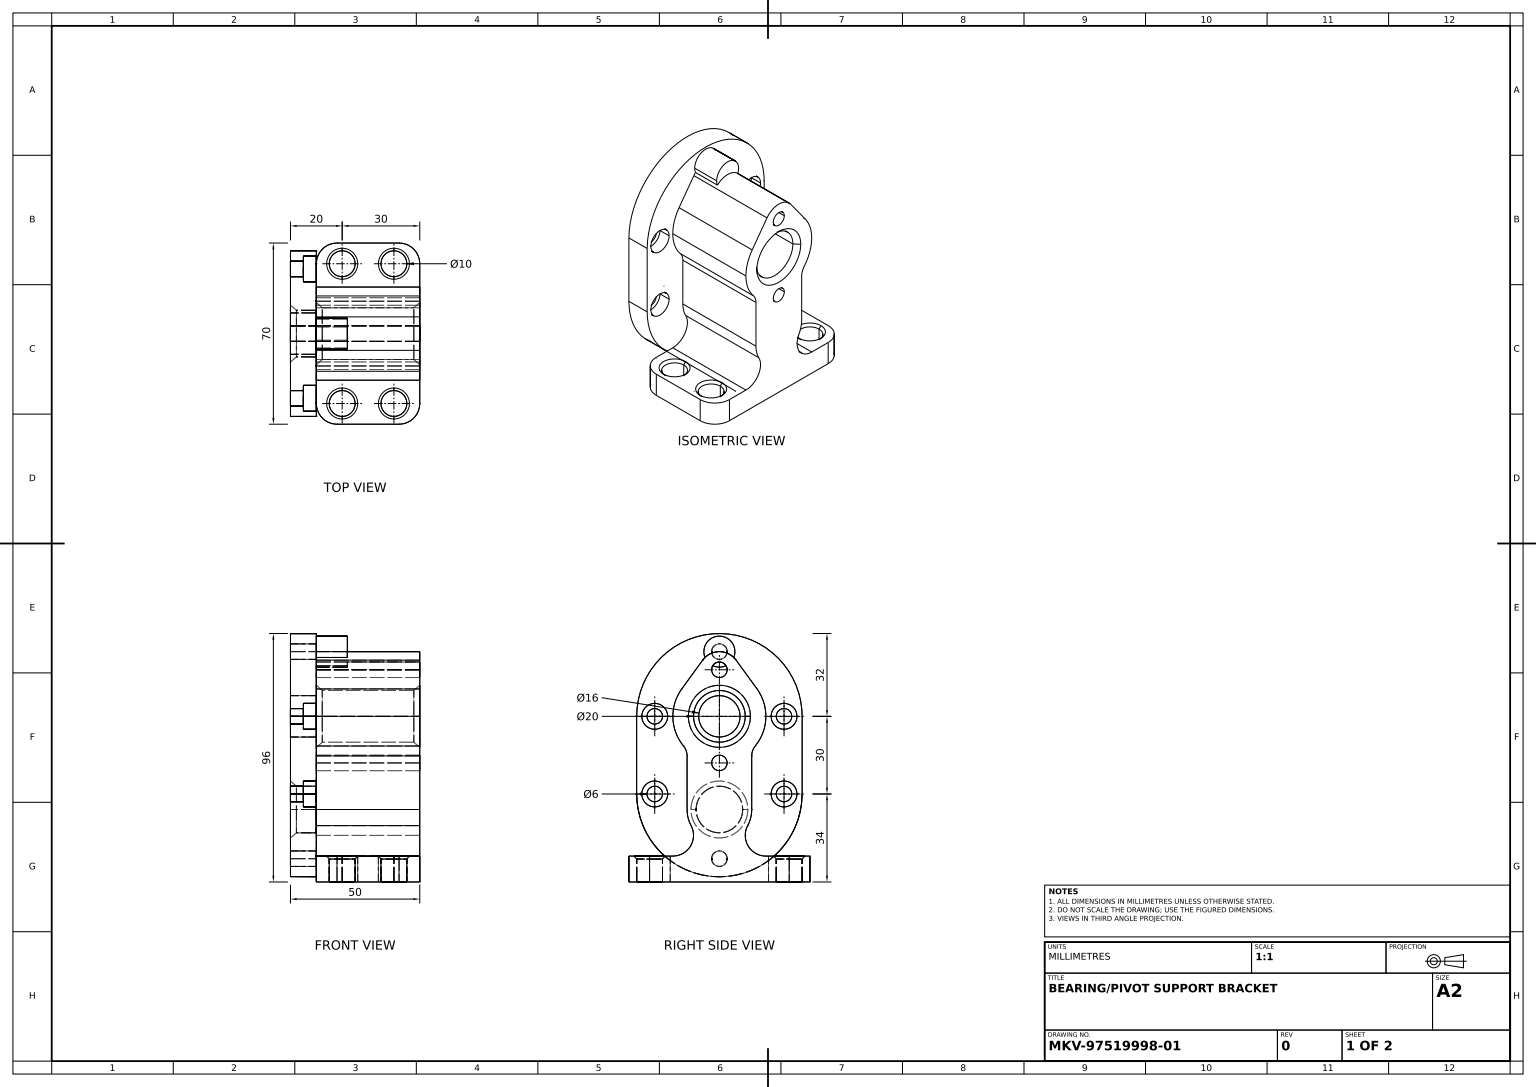
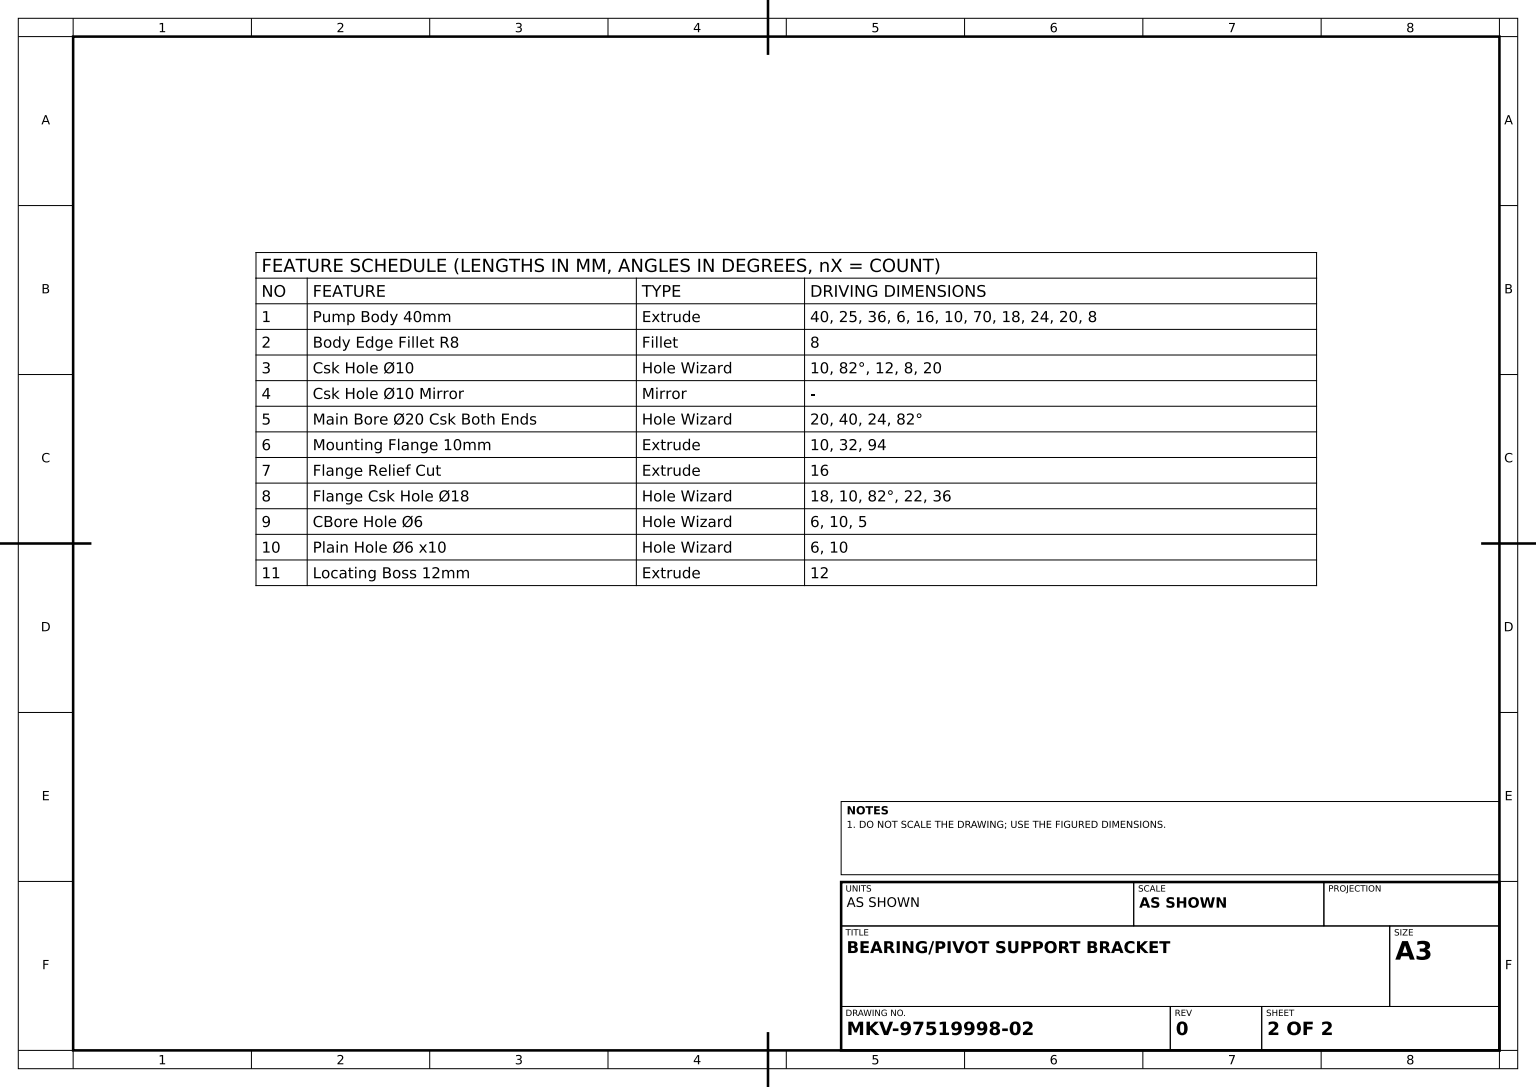
SolidWorks part; units mm, degrees
material "Plain Carbon Steel"
ref_plane "Front Plane" through (0, 0, 0) normal (0, 0, 1) x (1, 0, 0)
ref_plane "Top Plane" through (0, 0, 0) normal (0, 1, 0) x (1, 0, 0)
ref_plane "Right Plane" through (0, 0, 0) normal (1, 0, 0) x (0, 0, -1)
sketch "Body Profile Sketch" plane through (0, 0, 0) normal (1, 0, 0) x (0, 0, -1)
  line L0 (-12.5, -15.2889) -> (-12.5, -36)
  line L1 (12.5, -15.2889) -> (12.5, -36)
  line L2 (0, 0) -> (0, -6.2857) construction
  line L3 (-18, -54) -> (-35, -54)
  line L4 (-35, -54) -> (-35, -64)
  line L5 (-35, -64) -> (35, -64)
  line L6 (35, -64) -> (35, -54)
  line L7 (35, -54) -> (18, -54)
  line L8 (-14.5564, 10.5882) -> (-6.4695, 21.7059)
  line L9 (14.5564, 10.5882) -> (6.4695, 21.7059)
  arc A0 (13.875, -11.4667) -> (14.5564, 10.5882) centre (0, 0) ccw
  arc A1 (-12.5, -15.2889) -> (-13.875, -11.4667) centre (-18.5, -15.2889) ccw
  arc A2 (12.5, -15.2889) -> (13.875, -11.4667) centre (18.5, -15.2889) cw
  arc A3 (6.4695, 21.7059) -> (-6.4695, 21.7059) centre (0, 17) ccw
  arc A8 (-14.5564, 10.5882) -> (-13.875, -11.4667) centre (0, 0) ccw
  circle A10 centre (0, -36) radius 10 construction
  arc A11 (-12.5, -36) -> (-10.9412, -42.2353) centre (0.75, -36) ccw
  circle A12 centre (0, -36) radius 12 construction
  arc A13 (-18, -54) -> (-10.9412, -42.2353) centre (-18, -46) ccw
  arc A14 (12.5, -36) -> (10.9412, -42.2353) centre (-0.75, -36) cw
  arc A15 (18, -54) -> (10.9412, -42.2353) centre (18, -46) cw
  circle A16 centre (0, -18) radius 3
  circle A17 centre (0, 18) radius 3
  point P14 (0, 25)
  point P15 (0, -64)
  dimension "D1" = 18
  dimension "D4" = 6
  dimension "D5" = 16
  dimension "D8" = 24
  dimension "D9" = 25
  dimension "D11" = 20
  dimension "D12" = 8
  dimension "D13" = 6
  dimension "D15" = 6
  dimension "D2" = 25
  dimension "D3" = 36
  dimension "D6" = 10
  dimension "D7" = 70
  dimension "D10" = 18
  dimension "D14" = 18
  dimension "D16" = 18
  dimension "D17" = 36
extrude "Pump Body 40mm" add sketch "Body Profile Sketch" along normal blind 40
fillet "Body Edge Fillet R8" radius 8 4 edges at (0, -59, 35) (40, -59, 35) (0, -59, -35) (40, -59, -35)
hole_wizard "Csk Hole Ø10" positions "3DSketch2" profile "Sketch3" legacy end condition up to next
sketch3d "3DSketch2"
  line L1 (10, -54, 27) -> (52.0975, -54, 27) construction
  line L3 (32, -54, 35) -> (8, -54, 35) construction
  line L4 (40, -54, 18) -> (40, -54, 27) construction
  point P0 (10, -54, 27)
  point P2 (30, -54, 27)
  dimension "D1" = 8
  dimension "D2" = 20
  dimension "D3" = 10
sketch "Sketch3" plane through (10, -54, 27) normal (1, 0, 0) x (0, 0, 1)
  line L0 (0, 0) -> (0, 10)
  line L1 (0, 10) -> (5, 10)
  line L2 (5, 10) -> (5, 1.1504)
  line L3 (5, 1.1504) -> (6, 0)
  line L4 (6, 0) -> (0, 0)
  line L5 (0, -6.4453) -> (0, 115.525) construction
  line L6 (-5, 1.1504) -> (-6, 0) construction
  dimension "Diameter" = 10
  dimension "Depth" = 10
  dimension "C-Sink Angle" = 82
  dimension "C-Sink Diameter" = 12
mirror "Csk Hole Ø10 Mirror" about plane through (0, 0, 0) normal (0, 0, 1) of "Csk Hole Ø10"
hole_wizard "Main Bore Ø20 Csk Both Ends" positions "3DSketch3" profile "Sketch7" hole size "Ø20.0" standard "ISO" end condition up to next
sketch3d "3DSketch3"
  arc A3 (40, -11.4667, -13.875) -> (40, 10.5882, -14.5564) centre (40, 0, 0) ccw construction
  point P0 (0, 0, 0)
  point P3 (40, 0, 0)
  point P21 (58, 0, 0)
sketch "Sketch7" plane through (40, 0, 0) normal (0, 1, 0) x (0, 0, -1)
  line L0 (0, 0) -> (0, 40)
  line L1 (0, 40) -> (12, 40)
  line L2 (10, 37.6993) -> (10, 2.3007)
  line L3 (10, 2.3007) -> (12, 0)
  line L5 (12, 0) -> (0, 0)
  line L6 (-10, 2.3007) -> (-12, 0) construction
  line L7 (12, 40) -> (10, 37.6993)
  line L8 (-12, 40) -> (-10, 37.6993) construction
  line L11 (0, -6.35) -> (0, 107.95) construction
  dimension "Thru Hole Dia." = 20
  dimension "Thru Hole Depth" = 40
  dimension "Near C'Sink Dia." = 24
  dimension "Near C'Sink Angle" = 82
  dimension "Far C'Sink Dia." = 24
  dimension "Far C'Sink Angle" = 82
sketch "Mounting Flange Sketch" plane through (0, 0, 0) normal (-1, 0, 0) x (0, 0, 1)
  line L0 (0, 0) -> (0, -30) construction
  line L1 (32, 0) -> (32, -30)
  line L2 (-32, 0) -> (-32, -30)
  arc A0 (32, 0) -> (-32, 0) centre (0, 0) ccw
  arc A1 (-32, -30) -> (32, -30) centre (0, -30) ccw
  point P4 (0, -15)
  point P9 (0, 32)
  point P10 (0, -62)
  dimension "D2" = 32
  dimension "D1" = 94
extrude "Mounting Flange 10mm" add sketch "Mounting Flange Sketch" along normal blind 10
sketch "Flange Relief Cut Sketch" plane through (-10, 0, 0) normal (-1, 0, 0) x (0, 0, 1)
  circle A0 centre (0, 0) radius 8
  dimension "D1" = 16
extrude "Flange Relief Cut" cut sketch "Flange Relief Cut Sketch" against normal up to next
hole_wizard "Flange Csk Hole Ø18" positions "3DSketch4" profile "Sketch9" legacy
sketch3d "3DSketch4"
  line L1 (-10, -62, 0) -> (-10, 32, 0) construction
  line L2 (-10, 0, -32) -> (-10, 0, 32) construction
  arc A1 (-10, -30, -32) -> (-10, -30, 32) centre (-10, -30, 0) ccw construction
  arc A2 (-10, 0, 32) -> (-10, 0, -32) centre (-10, 0, 0) ccw construction
  point P0 (-10, -36, 0)
  point P17 (-42, -30, 0)
  point P21 (-42, 0, 0)
  dimension "D1" = 36
sketch "Sketch9" plane through (-10, -36, 0) normal (0, 1, 0) x (0, 0, 1)
  line L0 (0, 0) -> (0, 9.798)
  line L1 (0, 9.798) -> (9, 9.798)
  line L2 (9, 9.798) -> (9, 2.3007)
  line L3 (9, 2.3007) -> (11, 0)
  line L4 (11, 0) -> (0, 0)
  line L5 (0, -6.4453) -> (0, 115.525) construction
  line L6 (-9, 2.3007) -> (-11, 0) construction
  dimension "Diameter" = 18
  dimension "Depth" = 10
  dimension "C-Sink Angle" = 82
  dimension "C-Sink Diameter" = 22
sketch "Small Hole Layout Sketch" plane through (0, 0, 0) normal (-1, 0, 0) x (0, 0, 1)
  line L0 (0, 0) -> (0, -30) construction
  line L1 (25, 0) -> (25, -30)
  line L2 (-25, 0) -> (-25, -30)
  line L3 (32, 0) -> (32, -30) construction
  line L4 (11, -36) -> (0, -36) construction
  arc A0 (25, 0) -> (-25, 0) centre (0, 0) ccw
  arc A1 (-25, -30) -> (25, -30) centre (0, -30) ccw
  point P3 (0, -15)
  point P10 (32, -15)
  point P11 (0, 25)
  point P13 (0, -55)
  dimension "D1" = 19
hole_wizard "CBore Hole Ø6" positions "3DSketch6" profile "Sketch15" legacy end condition through all
sketch3d "3DSketch6"
  point P0 (0, -30, -25)
  point P3 (0, 0, -25)
  point P9 (0, -30, 25)
  point P12 (0, 0, 25)
sketch "Sketch15" plane through (0, -30, -25) normal (0, 1, 0) x (0, 0, -1)
  line L0 (0, 0) -> (0, 10)
  line L1 (0, 10) -> (3, 10)
  line L2 (3, 10) -> (3, 5)
  line L3 (3, 5) -> (5, 5)
  line L4 (5, 5) -> (5, 0)
  line L5 (5, 0) -> (0, 0)
  line L6 (0, 110) -> (0, -10) construction
  dimension "Diameter" = 6
  dimension "Depth" = 10
  dimension "C-Bore Diameter" = 10
  dimension "C-Bore Depth" = 5
hole_wizard "Plain Hole Ø6 x10" positions "3DSketch7" profile "Sketch16" legacy
sketch3d "3DSketch7"
  point P0 (0, -55, 0)
  point P4 (0, 25, 0)
sketch "Sketch16" plane through (0, -55, 0) normal (0, 1, 0) x (0, 0, -1)
  line L0 (0, 0) -> (0, 10)
  line L1 (0, 10) -> (3, 10)
  line L2 (3, 10) -> (3, 0)
  line L3 (3, 0) -> (0, 0)
  line L4 (0, 110) -> (0, -10) construction
  dimension "Diameter" = 6
  dimension "Depth" = 10
sketch "Locating Boss Sketch" plane through (0, 0, 0) normal (1, 0, 0) x (0, 0, -1)
  circle A0 centre (0, 25) radius 6
  arc A1 (6.4695, 21.7059) -> (-6.4695, 21.7059) centre (0, 17) ccw construction
  dimension "D1" = 12
extrude "Locating Boss 12mm" add sketch "Locating Boss Sketch" along normal blind 12
